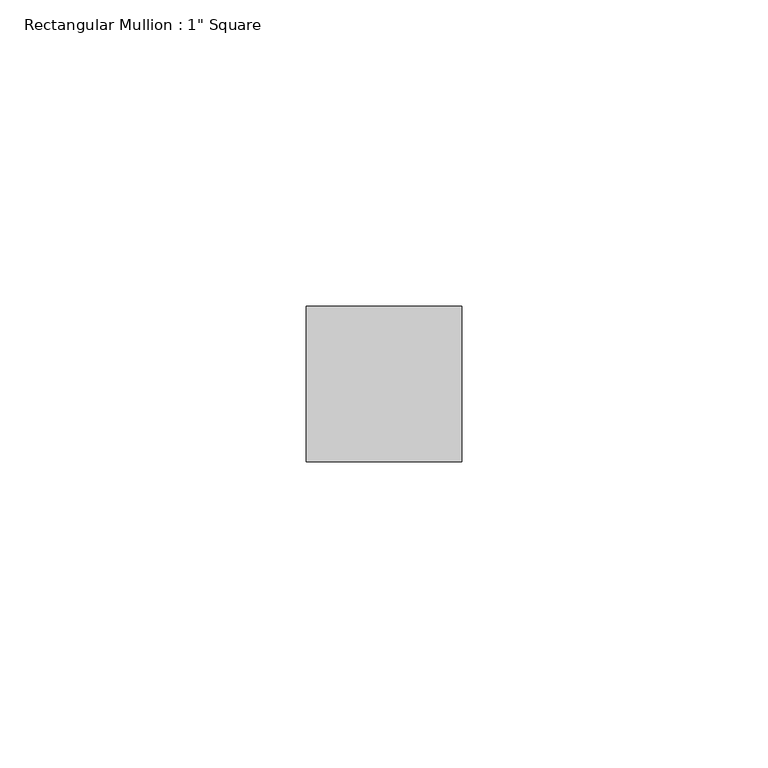
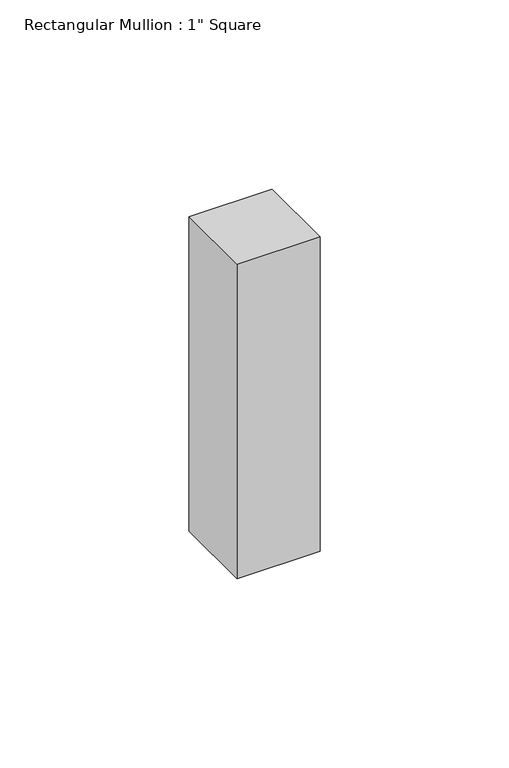
"""IFC4 building model written with IfcOpenShell, lengths in millimetres: member geometry."""

from ifc_helpers import new_model, si_unit, frame, origin, place, context, project, spatial, polyline, outline, extrude, source, transform, mapped, element, save


def member_d2c643f7(model_context):
    return source(origin(), model_context, "Body", "SweptSolid", [
        extrude(outline(polyline([(0.0, 12.7), (0.0, -12.7), (-25.4, -12.7), (-25.4, 12.7), (0.0, 12.7)])), frame((0.0, 0.0, -101.6), z_axis=(0.0, 0.0, 1.0), x_axis=(1.0, 0.0, 0.0)), (0.0, 0.0, 1.0), 101.6),
    ])


if __name__ == "__main__":
    model = new_model("IFC4")
    model_context = context("Model", 3, world=origin())
    ifc_project = project(units=[si_unit("LENGTHUNIT", "METRE", prefix="MILLI")], contexts=[model_context])
    site = spatial("IfcSite", under=ifc_project)
    building = spatial("IfcBuilding", under=site)
    placement = place(None, origin())
    member_shape = member_d2c643f7(model_context)
    element("IfcMember", 1, ObjectType="Rectangular Mullion : 1\" Square", at=placement, inside=building, context=model_context, shape_type="MappedRepresentation", body=[
        mapped(member_shape, transform((0.0, 0.0, 0.0), x_axis=(1.0, 0.0, 0.0), y_axis=(0.0, 1.0, 0.0), z_axis=(0.0, 0.0, 1.0))),
    ])
    save(model, "model.ifc")

# Revit data of these elements
# Type "Rectangular Mullion : 1\" Square"
#   built-in parameter 1007304 = 0.0833333 (stored number, unit not read)
#   built-in parameter 1007301 = 0.0416667 (stored number, unit not read)
#   built-in parameter 1007300 = 0.0416667 (stored number, unit not read)
